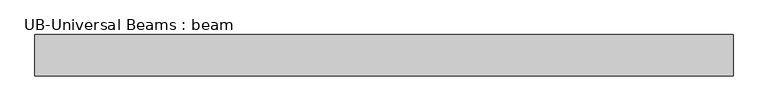
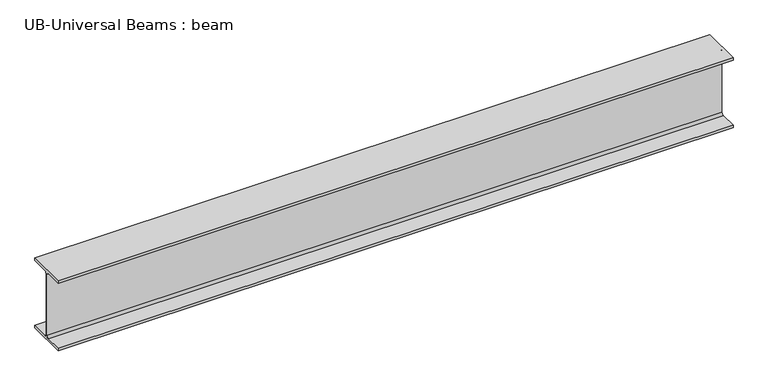
"""IFC4 building model written with IfcOpenShell, lengths in millimetres: beam geometry, UB-Universal Beams : beam."""

from ifc_helpers import new_model, si_unit, point, frame, frame_2d, origin, place, context, project, spatial, polyline, circle_curve, trimmed, segment, composite_curve, outline, extrude, source, transform, mapped, element, save


def ub_universal_beams_beam_d94dd637(model_context):
    return source(origin(), model_context, "Body", "SweptSolid", [
        extrude(outline(composite_curve([segment(polyline([(82.5, -141.5), (82.5, -151.7), (-82.5, -151.7), (-82.5, -141.5), (-11.9, -141.5)]), True, "CONTINUOUS"), segment(trimmed(circle_curve(frame_2d((-11.9, -132.6)), 8.9), [point((-11.9, -141.5))], [point((-3.0, -132.6))], True, "CARTESIAN"), True, "CONTINUOUS"), segment(polyline([(-3.0, -132.6), (-3.0, 132.6)]), True, "CONTINUOUS"), segment(trimmed(circle_curve(frame_2d((-11.9, 132.6)), 8.9), [point((-3.0, 132.6))], [point((-11.9, 141.5))], True, "CARTESIAN"), True, "CONTINUOUS"), segment(polyline([(-11.9, 141.5), (-82.5, 141.5), (-82.5, 151.7), (82.5, 151.7), (82.5, 141.5), (11.9, 141.5)]), True, "CONTINUOUS"), segment(trimmed(circle_curve(frame_2d((11.9, 132.6)), 8.9), [point((11.9, 141.5))], [point((3.0, 132.6))], True, "CARTESIAN"), True, "CONTINUOUS"), segment(polyline([(3.0, 132.6), (3.0, -132.6)]), True, "CONTINUOUS"), segment(trimmed(circle_curve(frame_2d((11.9, -132.6)), 8.9), [point((3.0, -132.6))], [point((11.9, -141.5))], True, "CARTESIAN"), True, "CONTINUOUS"), segment(polyline([(11.9, -141.5), (82.5, -141.5)]), True, "CONTINUOUS")], self_intersect=False)), frame((-1337.3, 0.0, 0.0), z_axis=(1.0, 0.0, 0.0), x_axis=(0.0, 1.0, 0.0)), (0.0, 0.0, 1.0), 2774.5),
    ])


if __name__ == "__main__":
    model = new_model("IFC4")
    model_context = context("Model", 3, world=origin())
    ifc_project = project(units=[si_unit("LENGTHUNIT", "METRE", prefix="MILLI")], contexts=[model_context])
    site = spatial("IfcSite", under=ifc_project)
    building = spatial("IfcBuilding", under=site)
    placement = place(None, origin())
    ub_universal_beams_beam_shape = ub_universal_beams_beam_d94dd637(model_context)
    element("IfcBeam", 1, ObjectType="UB-Universal Beams : beam", at=placement, inside=building, context=model_context, shape_type="MappedRepresentation", body=[
        mapped(ub_universal_beams_beam_shape, transform((0.0, 0.0, 0.0), x_axis=(1.0, 0.0, 0.0), y_axis=(0.0, 1.0, 0.0), z_axis=(0.0, 0.0, 1.0))),
    ])
    save(model, "model.ifc")

# Revit data of these elements
# Type "UB-Universal Beams : beam"
#   Section Name Key = "UB305X165X40"
#   Width = 16.5 cm
#   Web Thickness = 0.6 cm
#   Web Fillet = 0.89 cm
#   Warping Constant = 164000.0 cm⁶
#   Torsional Moment of Inertia = 14.70 cm⁴
#   Section Area = 51.3 cm²
#   Plastic Modulus weak axis = 142.0 cm³
#   Plastic Modulus strong axis = 623.0 cm³
#   Nominal Weight = 40.2999 kgf/m
#   Moment of Inertia weak axis = 764.00 cm⁴
#   Moment of Inertia strong axis = 8503.00 cm⁴
#   Height = 30.34 cm
#   Flange Thickness = 1.02 cm
#   Elastic Modulus weak axis = 92.6 cm³
#   Elastic Modulus strong axis = 560.0 cm³
#   Centroid Vertical = 15.17 cm
#   Centroid Horizontal = 8.25 cm
#   Bolt Spacing = 9.0 cm
#   Length [instance default] = 1.5 m
#   Structural Material [instance default] = Metal - Steel 43-275
#   Type Comments = ""
#   Assembly Code = ""
# Element 1 (IfcBeam, "UB-Universal Beams : beam")
#   Materials on its faces: "Metal - Steel 43-275"
# Materials
#   "Metal - Steel 43-275": class "Metal", colour RGB 247 247 247, transparency 0, Cost = 0
